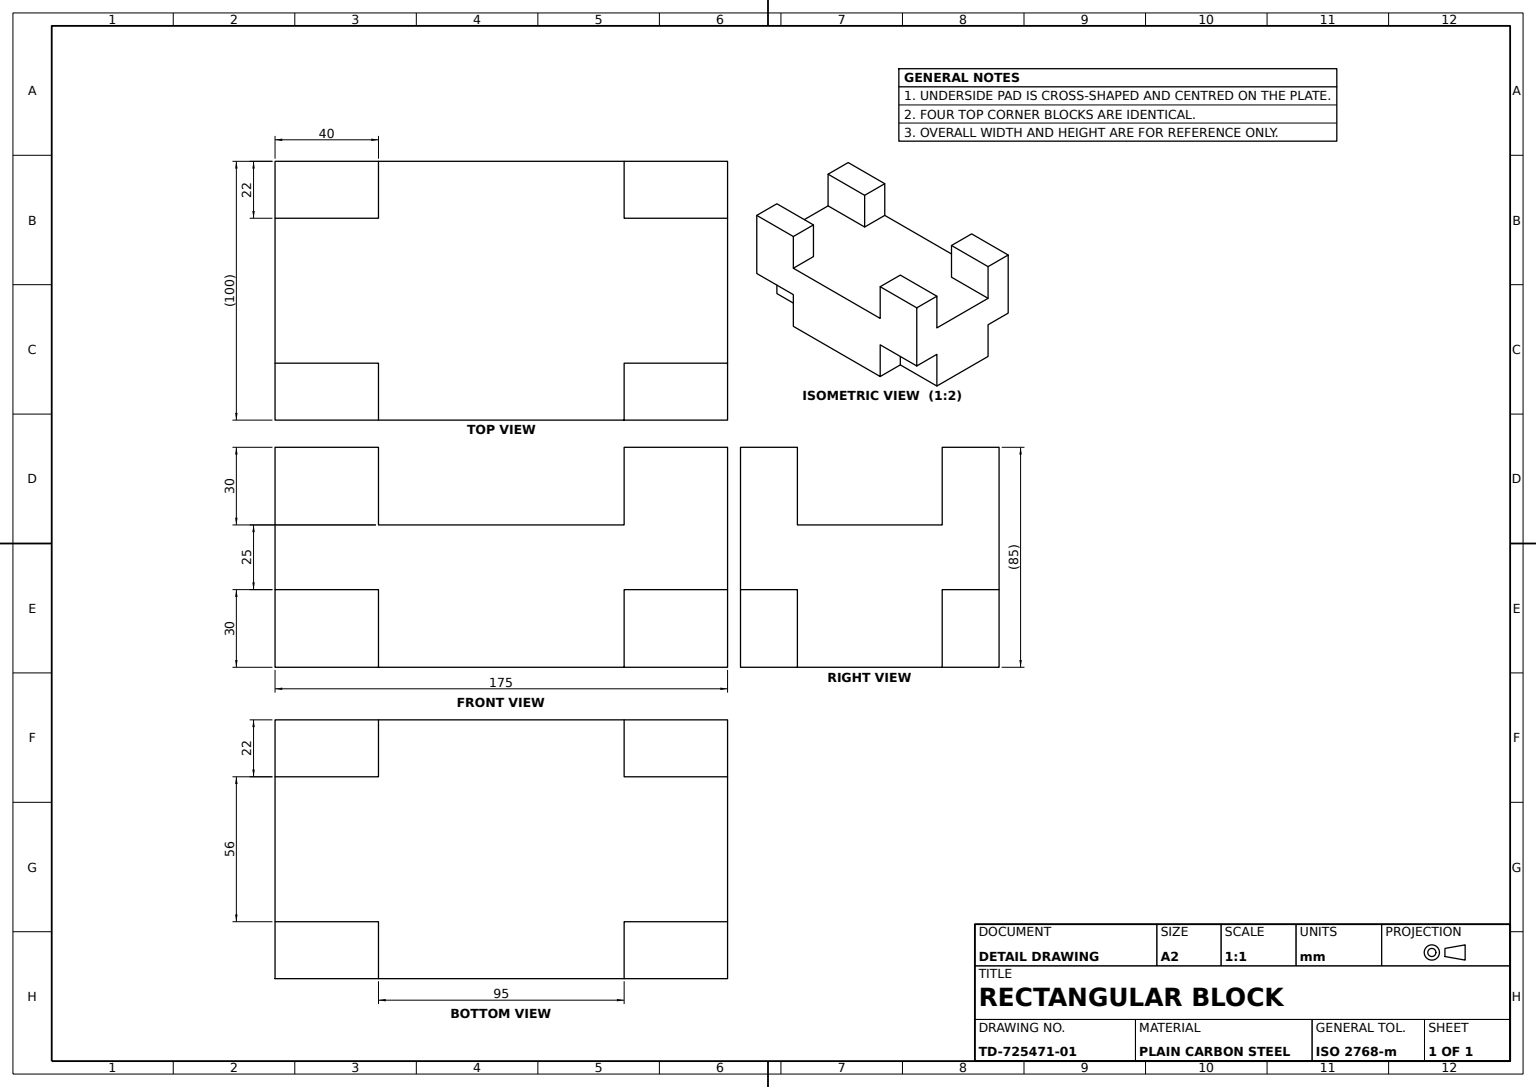
from build123d import *

# Parameters (mm, degrees)
BASE_PLATE_SKETCH_W         = 175
BASE_PLATE_SKETCH_H         = 100
BASE_PLATE_175X100X25_DEPTH = 25
TOP_BLOCKS_SKETCH_W         = 40
TOP_BLOCKS_SKETCH_H         = 22
TOP_BLOCKS_4X40X22_DEPTH    = 30
BOTTOM_PADS_DEPTH           = 30


with BuildPart() as part:
    # Base Plate Sketch → Base Plate 175x100x25 (new body)
    with BuildSketch(Plane(origin=(0, 0, 0), x_dir=(1, 0, 0), z_dir=(0, 1, 0))):
        Rectangle(BASE_PLATE_SKETCH_W, BASE_PLATE_SKETCH_H)
    extrude(amount=BASE_PLATE_175X100X25_DEPTH)

    # Top Blocks Sketch → Top Blocks 4x40x22 (add)
    with BuildSketch(Plane(origin=(0, 25, 0), x_dir=(1, 0, 0), z_dir=(0, 1, 0))):
        with Locations((-67.5, -39)):
            Rectangle(TOP_BLOCKS_SKETCH_W, TOP_BLOCKS_SKETCH_H)
        with Locations((-67.5, 39)):
            Rectangle(TOP_BLOCKS_SKETCH_W, TOP_BLOCKS_SKETCH_H)
        with Locations((67.5, 39)):
            Rectangle(TOP_BLOCKS_SKETCH_W, TOP_BLOCKS_SKETCH_H)
        with Locations((67.5, -39)):
            Rectangle(TOP_BLOCKS_SKETCH_W, TOP_BLOCKS_SKETCH_H)
    extrude(amount=TOP_BLOCKS_4X40X22_DEPTH)

    # Bottom Pads Sketch → Bottom Pads (add)
    with BuildSketch(Plane.XZ):
        Polygon((-47.5, 50), (47.5, 50), (47.5, 28), (87.5, 28), (87.5, -28), (47.5, -28), (47.5, -50), (-47.5, -50), (-47.5, -28), (-87.5, -28), (-87.5, 28), (-47.5, 28), align=None)
    extrude(amount=BOTTOM_PADS_DEPTH)


solid = part.part
